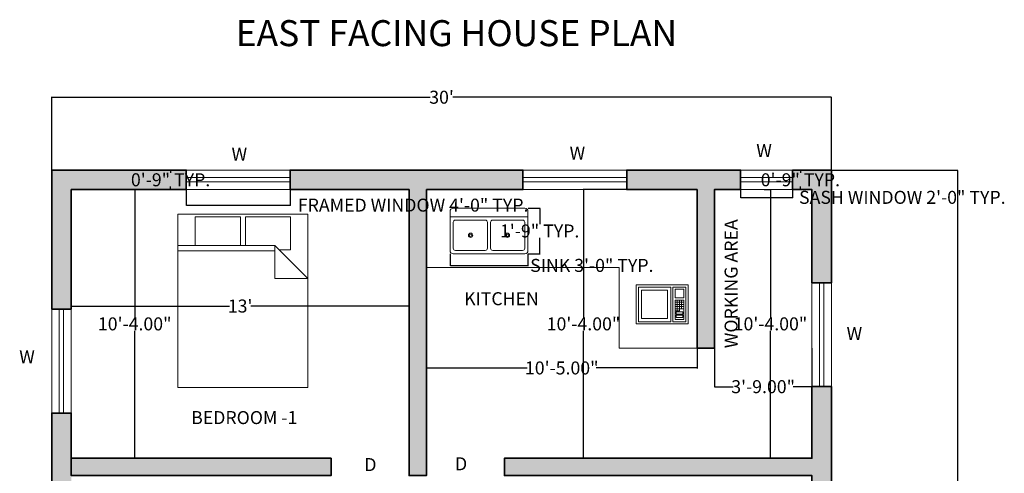
# Model space of a CAD drawing. Units: inches. Extents: x -977 to 1065, y -406 to 125.
# Tile 4 of 4: x 610 to 1065, y -89 to 121. Entities that reach past the tile are written whole.
import ezdxf

# ---------------------------------------------------------------- set-up
doc = ezdxf.new("R2010")
doc.units = ezdxf.units.IN
doc.header["$MEASUREMENT"] = 0
for name, color, linetype, lineweight in [('A-ANNO-DIMS', 2, 'Continuous', 13), ('A-ANNO-TEXT', 7, 'Continuous', 18), ('A-ANNO-TITL', 7, 'Continuous', 25), ('A-AREA-IDEN', 7, 'Continuous', 18), ('A-EQPM', 9, 'Continuous', 18), ('A-FLOR-CASE', 8, 'Continuous', 18), ('A-FLOR-FIXT', 8, 'Continuous', 18), ('A-FURN', 8, 'Continuous', 18), ('A-GLAZ', 5, 'Continuous', 18), ('A-WALL', 7, 'Continuous', 35), ('A-WALL-PATT', 252, 'Continuous', 13)]:
    doc.layers.add(name, color=color, linetype=linetype, lineweight=lineweight)
doc.styles.get("Standard").update_dxf_attribs({"font": 'arial.ttf'})
doc.dimstyles.get("Standard").update_dxf_attribs({"dimtxt": 6, "dimasz": 0.18, "dimexe": 0.18, "dimexo": 0.0625, "dimgap": 0.09, "dimtad": 0, "dimtih": 1, "dimtoh": 1, "dimzin": 0, "dimdsep": 46, "dimlunit": 3, "dimtxsty": 'Standard', "dimcen": 0.09, "dimadec": 0, "dimazin": 0, "dimtfac": 1, "dimtofl": 0, "dimtmove": 0, "dimatfit": 3, "dimfxl": 1, "dimtolj": 1, "dimtzin": 0, "dimarcsym": 0})

# ---------------------------------------------------------------- blocks, each defined once
blk = doc.blocks.new('Bed - Queen')
for p, q in [((0, -80.00003), (0, 0)), ((0, 0), (59.99999, 0)), ((59.99999, 0), (59.99999, -80.00003)), ((7.99999, -1.2), (28.79998, -1.2)), ((7.99999, -14.4), (7.99999, -1.2)), ((28.79998, -1.2), (28.79998, -14.4)), ((31.19999, -1.2), (51.99999, -1.2)), ((31.19999, -14.4), (31.19999, -1.2)), ((51.99999, -1.2), (51.99999, -16.4)), ((0, -14.4), (44.8, -14.4)), ((44.8, -16.8), (0, -16.8)), ((59.99999, -29.6), (44.8, -14.4)), ((44.8, -14.4), (44.8, -29.6)), ((51.99999, -16.4), (46.79936, -16.4)), ((44.8, -29.6), (59.99999, -29.6)), ((59.99999, -80.00003), (0, -80.00003))]:
    blk.add_line(p, q)
blk = doc.blocks.new('Sink-double - 36 in top')
for p, q in [((-18, -4), (18, -4)), ((-0.75, -18.5), (-0.75, -6.5)), ((0.75, -6.5), (0.75, -18.5))]:
    blk.add_line(p, q)
for points in [[(-16.5, 0), (16.5, 0)], [(-18, -19.5), (-18, -1.5)], [(18, -1.5), (18, -19.5)], [(-16.5, -18.5), (-16.5, -6.5)], [(-15.5, -5.5), (-1.75, -5.5)], [(1.75, -5.5), (15.5, -5.5)], [(16.5, -6.5), (16.5, -18.5)], [(16.5, -21), (-16.5, -21)], [(-1.75, -19.5), (-15.5, -19.5)], [(15.5, -19.5), (1.75, -19.5)]]:
    blk.add_lwpolyline(points)
for centre, radius in [((-8.5, -12.5), 1), ((-8.5, -12.5), 0.5), ((8.5, -12.5), 1), ((8.5, -12.5), 0.5)]:
    blk.add_circle(centre, radius)
for centre, radius, start, end in [((-16.5, -1.5), 1.5, 90, 180), ((16.5, -1.5), 1.5, 0, 90), ((-15.5, -6.5), 1, 90, 180), ((-1.75, -6.5), 1, 0, 90), ((1.75, -6.5), 1, 90, 180), ((15.5, -6.5), 1, 0, 90), ((-16.5, -19.5), 1.5, 180, 270), ((-15.5, -18.5), 1, 180, 270), ((-1.75, -18.5), 1, 270, 0), ((1.75, -18.5), 1, 180, 270), ((15.5, -18.5), 1, 270, 0), ((16.5, -19.5), 1.5, 270, 0)]:
    blk.add_arc(centre, radius, start, end)
blk = doc.blocks.new('Microwave')
for p, q in [((18, 10), (22, 10)), ((19, 7), (19, 11)), ((20, 11), (20, 7)), ((21, 7), (21, 11)), ((22, 9), (18, 9)), ((18, 8), (22, 8)), ((22, 7), (18, 7)), ((20, 6), (18, 6)), ((19, 6), (19, 7)), ((20, 7), (20, 6))]:
    blk.add_line(p, q)
for points in [[(0, 0), (0, 18), (24, 18), (24, 0)], [(1, 1), (1, 17), (16, 17), (16, 1)], [(2.5, 2.5), (2.5, 15.5), (14.5, 15.5), (14.5, 2.5)], [(17, 1), (17, 17), (23, 17), (23, 1)], [(18, 12), (18, 16), (22, 16), (22, 12)], [(18, 2), (18, 11), (22, 11), (22, 2)], [(18.5, 4.5), (18.5, 5.5), (21.5, 5.5), (21.5, 4.5)], [(18.5, 3), (18.5, 4), (21.5, 4), (21.5, 3)]]:
    blk.add_lwpolyline(points, close=True)
blk = doc.blocks.new('*D31')
at = {"layer": 'A-ANNO-DIMS', "color": 0, "lineweight": -2, "transparency": 16777216}
for p, q in [((625.09, 51.05), (625.09, 85.12)), ((625.27, 84.94), (799.91, 84.94)), ((984.91, 84.94), (810.27, 84.94)), ((985.09, 51.4), (985.09, 85.12))]:
    blk.add_line(p, q, dxfattribs=at)
at = {"layer": 'A-ANNO-DIMS', "color": 0, "transparency": 16777216}
for points in [[(625.27, 84.97), (625.27, 84.91), (625.09, 84.94)], [(984.91, 84.97), (984.91, 84.91), (985.09, 84.94)]]:
    blk.add_solid(points, dxfattribs=at)
at = {"layer": 'Defpoints', "color": 0, "transparency": 16777216}
for p in [(985.09, 84.94), (625.09, 50.99), (985.09, 51.33)]:
    blk.add_point(p, dxfattribs=at)
at = {"layer": 'A-ANNO-DIMS', "color": 0, "transparency": 16777216, "insert": (805.09, 84.94), "char_height": 6, "attachment_point": 5}
blk.add_mtext("\\A1;30'", dxfattribs=at)
blk = doc.blocks.new('*D32')
at = {"layer": 'A-ANNO-DIMS', "color": 0, "lineweight": -2, "transparency": 16777216}
for p, q in [((985.15, 51.33), (1043.56, 51.33)), ((1043.38, 51.15), (1043.38, -167.51)), ((1043.38, -392.49), (1043.38, -173.82)), ((985.15, -392.67), (1043.56, -392.67))]:
    blk.add_line(p, q, dxfattribs=at)
at = {"layer": 'A-ANNO-DIMS', "color": 0, "transparency": 16777216}
for points in [[(1043.35, 51.15), (1043.41, 51.15), (1043.38, 51.33)], [(1043.35, -392.49), (1043.41, -392.49), (1043.38, -392.67)]]:
    blk.add_solid(points, dxfattribs=at)
at = {"layer": 'Defpoints', "color": 0, "transparency": 16777216}
for p in [(985.09, 51.33), (985.09, -392.67), (1043.38, -392.67)]:
    blk.add_point(p, dxfattribs=at)
at = {"layer": 'A-ANNO-DIMS', "color": 0, "transparency": 16777216, "insert": (1043.38, -170.67), "char_height": 6, "attachment_point": 5}
blk.add_mtext("\\A1;37'", dxfattribs=at)
blk = doc.blocks.new('*D33')
at = {"layer": 'A-ANNO-DIMS', "color": 0, "lineweight": -2, "transparency": 16777216}
for p, q in [((634.09, -3.08), (634.09, -11.62)), ((790.09, -3.08), (790.09, -11.62)), ((634.27, -11.44), (707.19, -11.44)), ((789.91, -11.44), (716.99, -11.44))]:
    blk.add_line(p, q, dxfattribs=at)
at = {"layer": 'A-ANNO-DIMS', "color": 0, "transparency": 16777216}
for points in [[(634.27, -11.41), (634.27, -11.47), (634.09, -11.44)], [(789.91, -11.41), (789.91, -11.47), (790.09, -11.44)]]:
    blk.add_solid(points, dxfattribs=at)
at = {"layer": 'Defpoints', "color": 0, "transparency": 16777216}
for p in [(634.09, -3.02), (790.09, -3.02), (790.09, -11.44)]:
    blk.add_point(p, dxfattribs=at)
at = {"layer": 'A-ANNO-DIMS', "color": 0, "transparency": 16777216, "insert": (712.09, -11.44), "char_height": 6, "attachment_point": 5}
blk.add_mtext("\\A1;13'", dxfattribs=at)
blk = doc.blocks.new('*D34')
at = {"layer": 'A-ANNO-DIMS', "color": 0, "lineweight": -2, "transparency": 16777216}
for p, q in [((668.37, 42.33), (663.23, 42.33)), ((663.41, 42.15), (663.41, -16.51)), ((663.41, -81.49), (663.41, -22.82)), ((668.37, -81.67), (663.23, -81.67))]:
    blk.add_line(p, q, dxfattribs=at)
at = {"layer": 'A-ANNO-DIMS', "color": 0, "transparency": 16777216}
for points in [[(663.38, 42.15), (663.44, 42.15), (663.41, 42.33)], [(663.38, -81.49), (663.44, -81.49), (663.41, -81.67)]]:
    blk.add_solid(points, dxfattribs=at)
at = {"layer": 'Defpoints', "color": 0, "transparency": 16777216}
for p in [(668.43, 42.33), (663.41, -81.67), (668.43, -81.67)]:
    blk.add_point(p, dxfattribs=at)
at = {"layer": 'A-ANNO-DIMS', "color": 0, "transparency": 16777216, "insert": (663.41, -19.67), "char_height": 6, "attachment_point": 5}
blk.add_mtext('\\A1;10\'-4.00"', dxfattribs=at)
blk = doc.blocks.new('*D37')
at = {"layer": 'A-ANNO-DIMS', "color": 0, "lineweight": -2, "transparency": 16777216}
for p, q in [((798.09, 6.27), (798.09, -40.2)), ((923.09, 5.65), (923.09, -40.2)), ((798.27, -40.02), (844.65, -40.02)), ((922.91, -40.02), (876.53, -40.02))]:
    blk.add_line(p, q, dxfattribs=at)
at = {"layer": 'A-ANNO-DIMS', "color": 0, "transparency": 16777216}
for points in [[(798.27, -39.99), (798.27, -40.05), (798.09, -40.02)], [(922.91, -39.99), (922.91, -40.05), (923.09, -40.02)]]:
    blk.add_solid(points, dxfattribs=at)
at = {"layer": 'Defpoints', "color": 0, "transparency": 16777216}
for p in [(798.09, 6.33), (923.09, 5.72), (923.09, -40.02)]:
    blk.add_point(p, dxfattribs=at)
at = {"layer": 'A-ANNO-DIMS', "color": 0, "transparency": 16777216, "insert": (860.59, -40.02), "char_height": 6, "attachment_point": 5}
blk.add_mtext('\\A1;10\'-5.00"', dxfattribs=at)
blk = doc.blocks.new('*D38')
at = {"layer": 'A-ANNO-DIMS', "color": 0, "lineweight": -2, "transparency": 16777216}
for p, q in [((901.19, 42.33), (870.46, 42.33)), ((870.64, 42.15), (870.64, -16.51)), ((870.64, -81.49), (870.64, -22.82)), ((901.19, -81.67), (870.46, -81.67))]:
    blk.add_line(p, q, dxfattribs=at)
at = {"layer": 'A-ANNO-DIMS', "color": 0, "transparency": 16777216}
for points in [[(870.61, 42.15), (870.67, 42.15), (870.64, 42.33)], [(870.61, -81.49), (870.67, -81.49), (870.64, -81.67)]]:
    blk.add_solid(points, dxfattribs=at)
at = {"layer": 'Defpoints', "color": 0, "transparency": 16777216}
for p in [(901.25, 42.33), (870.64, -81.67), (901.25, -81.67)]:
    blk.add_point(p, dxfattribs=at)
at = {"layer": 'A-ANNO-DIMS', "color": 0, "transparency": 16777216, "insert": (870.64, -19.67), "char_height": 6, "attachment_point": 5}
blk.add_mtext('\\A1;10\'-4.00"', dxfattribs=at)
blk = doc.blocks.new('*D39')
at = {"layer": 'A-ANNO-DIMS', "color": 0, "lineweight": -2, "transparency": 16777216}
for p, q in [((954.03, 42.33), (957.16, 42.33)), ((956.98, 42.15), (956.98, -16.51)), ((956.98, -81.49), (956.98, -22.82)), ((954.03, -81.67), (957.16, -81.67))]:
    blk.add_line(p, q, dxfattribs=at)
at = {"layer": 'A-ANNO-DIMS', "color": 0, "transparency": 16777216}
for points in [[(956.95, 42.15), (957.01, 42.15), (956.98, 42.33)], [(956.95, -81.49), (957.01, -81.49), (956.98, -81.67)]]:
    blk.add_solid(points, dxfattribs=at)
at = {"layer": 'Defpoints', "color": 0, "transparency": 16777216}
for p in [(953.97, 42.33), (953.97, -81.67), (956.98, -81.67)]:
    blk.add_point(p, dxfattribs=at)
at = {"layer": 'A-ANNO-DIMS', "color": 0, "transparency": 16777216, "insert": (956.98, -19.67), "char_height": 6, "attachment_point": 5}
blk.add_mtext('\\A1;10\'-4.00"', dxfattribs=at)
blk = doc.blocks.new('*D40')
at = {"layer": 'A-ANNO-DIMS', "color": 0, "lineweight": -2, "transparency": 16777216}
for p, q in [((931.09, -30.96), (931.09, -48.84)), ((976.09, -30.96), (976.09, -48.84)), ((931.27, -48.66), (939.7, -48.66)), ((975.91, -48.66), (967.48, -48.66))]:
    blk.add_line(p, q, dxfattribs=at)
at = {"layer": 'A-ANNO-DIMS', "color": 0, "transparency": 16777216}
for points in [[(931.27, -48.63), (931.27, -48.69), (931.09, -48.66)], [(975.91, -48.63), (975.91, -48.69), (976.09, -48.66)]]:
    blk.add_solid(points, dxfattribs=at)
at = {"layer": 'Defpoints', "color": 0, "transparency": 16777216}
for p in [(931.09, -30.9), (976.09, -30.9), (976.09, -48.66)]:
    blk.add_point(p, dxfattribs=at)
at = {"layer": 'A-ANNO-DIMS', "color": 0, "transparency": 16777216, "insert": (953.59, -48.66), "char_height": 6, "attachment_point": 5}
blk.add_mtext('\\A1;3\'-9.00"', dxfattribs=at)
blk = doc.blocks.new('WIN-48-FRAMED')
for p, q in [((0, 48), (9, 48)), ((0, 0), (0, 48)), ((3.5, 0), (3.5, 48)), ((5.5, 48), (5.5, 0)), ((9, 48), (9, 0)), ((9, 0), (0, 0))]:
    blk.add_line(p, q)
for points in [[(0, 0), (0, 48)], [(9, 0), (9, 48)]]:
    blk.add_lwpolyline(points)
blk = doc.blocks.new('WIN-24-SASH')
for p, q in [((0, 5.5), (24, 5.5)), ((24, 9), (24, 0)), ((24, 3.5), (0, 3.5)), ((24, 0), (0, 0))]:
    blk.add_line(p, q)
for points in [[(0, 9), (24, 9)], [(0, 0), (24, 0)]]:
    blk.add_lwpolyline(points)
blk = doc.blocks.new('*D52')
at = {"layer": 'A-ANNO-DIMS', "color": 0, "lineweight": -2, "transparency": 16777216}
for p, q in [((687.18, 42.27), (687.18, 34.95)), ((735.18, 42.27), (735.18, 34.95)), ((687.36, 35.13), (735, 35.13)), ((735.18, 35.13), (735.36, 35.13))]:
    blk.add_line(p, q, dxfattribs=at)
at = {"layer": 'A-ANNO-DIMS', "color": 0, "transparency": 16777216}
for points in [[(687.36, 35.16), (687.36, 35.1), (687.18, 35.13)], [(735, 35.16), (735, 35.1), (735.18, 35.13)]]:
    blk.add_solid(points, dxfattribs=at)
at = {"layer": 'Defpoints', "color": 0, "transparency": 16777216}
for p in [(687.18, 42.33), (735.18, 42.33), (735.18, 35.13)]:
    blk.add_point(p, dxfattribs=at)
at = {"layer": 'A-ANNO-DIMS', "color": 0, "transparency": 16777216, "insert": (791.98, 35.13), "char_height": 6, "attachment_point": 5}
blk.add_mtext('\\A1;FRAMED WINDOW 4\'-0" TYP.', dxfattribs=at)
blk = doc.blocks.new('*D53')
at = {"layer": 'A-ANNO-DIMS', "color": 0, "lineweight": -2, "transparency": 16777216}
for p, q in [((687.12, 51.33), (679.8, 51.33)), ((679.98, 51.15), (679.98, 49.99)), ((687.12, 42.33), (679.8, 42.33)), ((679.98, 42.51), (679.98, 43.68))]:
    blk.add_line(p, q, dxfattribs=at)
at = {"layer": 'A-ANNO-DIMS', "color": 0, "transparency": 16777216}
for points in [[(679.95, 51.15), (680.01, 51.15), (679.98, 51.33)], [(679.95, 42.51), (680.01, 42.51), (679.98, 42.33)]]:
    blk.add_solid(points, dxfattribs=at)
at = {"layer": 'Defpoints', "color": 0, "transparency": 16777216}
for p in [(687.18, 51.33), (679.98, 42.33), (687.18, 42.33)]:
    blk.add_point(p, dxfattribs=at)
at = {"layer": 'A-ANNO-DIMS', "color": 0, "transparency": 16777216, "insert": (679.98, 46.83), "char_height": 6, "attachment_point": 5}
blk.add_mtext('\\A1;0\'-9" TYP.', dxfattribs=at)
blk = doc.blocks.new('*D58')
at = {"layer": 'A-ANNO-DIMS', "color": 0, "lineweight": -2, "transparency": 16777216}
for p, q in [((943.18, 42.27), (943.18, 38.55)), ((967.18, 42.27), (967.18, 38.55)), ((943.36, 38.73), (967, 38.73)), ((967.18, 38.73), (967.36, 38.73))]:
    blk.add_line(p, q, dxfattribs=at)
at = {"layer": 'A-ANNO-DIMS', "color": 0, "transparency": 16777216}
for points in [[(943.36, 38.76), (943.36, 38.7), (943.18, 38.73)], [(967, 38.76), (967, 38.7), (967.18, 38.73)]]:
    blk.add_solid(points, dxfattribs=at)
at = {"layer": 'Defpoints', "color": 0, "transparency": 16777216}
for p in [(943.18, 42.33), (967.18, 42.33), (967.18, 38.73)]:
    blk.add_point(p, dxfattribs=at)
at = {"layer": 'A-ANNO-DIMS', "color": 0, "transparency": 16777216, "insert": (1017.85, 38.73), "char_height": 6, "attachment_point": 5}
blk.add_mtext('\\A1;SASH WINDOW 2\'-0" TYP.', dxfattribs=at)
blk = doc.blocks.new('*D59')
at = {"layer": 'A-ANNO-DIMS', "color": 0, "lineweight": -2, "transparency": 16777216}
for p, q in [((967.24, 51.33), (970.96, 51.33)), ((970.78, 51.15), (970.78, 49.99)), ((967.24, 42.33), (970.96, 42.33)), ((970.78, 42.51), (970.78, 43.68))]:
    blk.add_line(p, q, dxfattribs=at)
at = {"layer": 'A-ANNO-DIMS', "color": 0, "transparency": 16777216}
for points in [[(970.75, 51.15), (970.81, 51.15), (970.78, 51.33)], [(970.75, 42.51), (970.81, 42.51), (970.78, 42.33)]]:
    blk.add_solid(points, dxfattribs=at)
at = {"layer": 'Defpoints', "color": 0, "transparency": 16777216}
for p in [(967.18, 51.33), (970.78, 51.33), (967.18, 42.33)]:
    blk.add_point(p, dxfattribs=at)
at = {"layer": 'A-ANNO-DIMS', "color": 0, "transparency": 16777216, "insert": (970.78, 46.83), "char_height": 6, "attachment_point": 5}
blk.add_mtext('\\A1;0\'-9" TYP.', dxfattribs=at)
blk = doc.blocks.new('*D60')
at = {"layer": 'A-ANNO-DIMS', "color": 0, "lineweight": -2, "transparency": 16777216}
for p, q in [((809.01, 12.65), (809.01, 7.13)), ((845.01, 12.65), (845.01, 7.13)), ((809.19, 7.31), (844.83, 7.31)), ((845.01, 7.31), (845.19, 7.31))]:
    blk.add_line(p, q, dxfattribs=at)
at = {"layer": 'A-ANNO-DIMS', "color": 0, "transparency": 16777216}
for points in [[(809.19, 7.34), (809.19, 7.28), (809.01, 7.31)], [(844.83, 7.34), (844.83, 7.28), (845.01, 7.31)]]:
    blk.add_solid(points, dxfattribs=at)
at = {"layer": 'Defpoints', "color": 0, "transparency": 16777216}
for p in [(809.01, 12.71), (845.01, 12.71), (845.01, 7.31)]:
    blk.add_point(p, dxfattribs=at)
at = {"layer": 'A-ANNO-DIMS', "color": 0, "transparency": 16777216, "insert": (874.5, 7.31), "char_height": 6, "attachment_point": 5}
blk.add_mtext('\\A1;SINK 3\'-0" TYP.', dxfattribs=at)
blk = doc.blocks.new('*D61')
at = {"layer": 'A-ANNO-DIMS', "color": 0, "lineweight": -2, "transparency": 16777216}
for p, q in [((845.07, 33.71), (850.59, 33.71)), ((850.41, 33.53), (850.41, 26.36)), ((850.41, 12.89), (850.41, 20.06)), ((845.07, 12.71), (850.59, 12.71))]:
    blk.add_line(p, q, dxfattribs=at)
at = {"layer": 'A-ANNO-DIMS', "color": 0, "transparency": 16777216}
for points in [[(850.38, 33.53), (850.44, 33.53), (850.41, 33.71)], [(850.38, 12.89), (850.44, 12.89), (850.41, 12.71)]]:
    blk.add_solid(points, dxfattribs=at)
at = {"layer": 'Defpoints', "color": 0, "transparency": 16777216}
for p in [(845.01, 33.71), (850.41, 33.71), (845.01, 12.71)]:
    blk.add_point(p, dxfattribs=at)
at = {"layer": 'A-ANNO-DIMS', "color": 0, "transparency": 16777216, "insert": (850.41, 23.21), "char_height": 6, "attachment_point": 5}
blk.add_mtext('\\A1;1\'-9" TYP.', dxfattribs=at)

msp = doc.modelspace()

# ---------------------------------------------------------------- hatches: boundary and pattern name
at = {"layer": 'A-WALL-PATT'}
h = msp.add_hatch(color=256, dxfattribs=at)
h.dxf.hatch_style = 1
h.paths.add_polyline_path([(637.06, 42.333), (687.18, 42.333), (687.18, 51.333), (625.089, 51.333), (625.089, -12.85), (634.089, -12.85), (634.089, 42.333)])
h = msp.add_hatch(color=256, dxfattribs=at)
h.dxf.hatch_style = 1
h.paths.add_polyline_path([(798.089, 42.333), (798.089, -89.667), (790.089, -89.667), (790.089, 42.333), (735.18, 42.333), (735.18, 51.333), (842.634, 51.333), (842.634, 42.333)])
h = msp.add_hatch(color=256, dxfattribs=at)
h.dxf.hatch_style = 1
h.paths.add_polyline_path([(943.182, 42.333), (943.182, 51.333), (890.634, 51.333), (890.634, 42.333), (923.089, 42.333), (923.089, -30.9), (931.089, -30.9), (931.089, 42.333)])
h = msp.add_hatch(color=256, dxfattribs=at)
h.dxf.hatch_style = 1
h.paths.add_polyline_path([(985.089, -0.655), (985.089, 51.333), (967.182, 51.333), (967.182, 42.333), (976.089, 42.333), (976.089, -0.655)])
h = msp.add_hatch(color=256, dxfattribs=at)
h.dxf.hatch_style = 1
h.paths.add_polyline_path([(985.089, -125.667), (985.089, -48.655), (976.089, -48.655), (976.089, -81.667), (834.089, -81.667), (834.089, -89.667), (976.089, -89.667), (976.089, -125.667)])
h = msp.add_hatch(color=256, dxfattribs=at)
h.dxf.hatch_style = 1
h.paths.add_polyline_path([(625.089, -109.279), (625.089, -60.85), (634.089, -60.85), (634.089, -109.279)])
h = msp.add_hatch(color=256, dxfattribs=at)
h.dxf.hatch_style = 1
h.paths.add_polyline_path([(754.089, -81.667), (634.089, -81.667), (634.089, -89.667), (754.089, -89.667)])

# ---------------------------------------------------------------- linework, layer by layer
at = {"layer": 'A-FLOR-CASE'}
msp.add_line((887.089, -30.9), (923.089, -30.9), dxfattribs=at)
for points in [[(798.089, 6.333), (887.089, 6.333)], [(887.089, -30.9), (887.089, 6.333)]]:
    msp.add_lwpolyline(points, dxfattribs=at)
at = {"layer": 'A-GLAZ'}
for p, q in [((943.182, 51.333), (967.182, 51.333)), ((735.18, 42.333), (735.18, 46.833))]:
    msp.add_line(p, q, dxfattribs=at)
at = {"layer": 'A-WALL'}
for points in [[(637.06, 42.333), (687.18, 42.333), (687.18, 51.333), (625.089, 51.333), (625.089, -12.85), (634.089, -12.85), (634.089, 42.333)], [(798.089, 42.333), (798.089, -89.667), (790.089, -89.667), (790.089, 42.333), (735.18, 42.333), (735.18, 51.333), (842.634, 51.333), (842.634, 42.333)], [(943.182, 42.333), (943.182, 51.333), (890.634, 51.333), (890.634, 42.333), (923.089, 42.333), (923.089, -30.9), (931.089, -30.9), (931.089, 42.333)], [(985.089, -0.655), (985.089, 51.333), (967.182, 51.333), (967.182, 42.333), (976.089, 42.333), (976.089, -0.655)], [(754.089, -81.667), (634.089, -81.667), (634.089, -89.667), (754.089, -89.667)]]:
    msp.add_lwpolyline(points, close=True, dxfattribs=at)
for points in [[(985.089, -125.667), (985.089, -48.655), (976.089, -48.655), (976.089, -81.667), (834.089, -81.667), (834.089, -89.667), (976.089, -89.667), (976.089, -125.667), (985.089, -125.667), (985.089, -116.301)], [(625.089, -109.279), (625.089, -60.85), (634.089, -60.85), (634.089, -81.667)]]:
    msp.add_lwpolyline(points, dxfattribs=at)

# ---------------------------------------------------------------- block references
at = {"layer": 'A-EQPM'}
msp.add_blockref('Microwave', (894.96, -19.685), dxfattribs=at)
at = {"layer": 'A-FLOR-FIXT'}
msp.add_blockref('Sink-double - 36 in top', (827.01, 33.711), dxfattribs=at)
at = {"layer": 'A-FURN'}
msp.add_blockref('Bed - Queen', (683.391, 30.912), dxfattribs=at)
at = {"layer": 'A-GLAZ'}
for p, rotation in [((687.18, 51.333), 269.9999999999999), ((842.634, 51.333), 270), ((985.089, -0.655), 180)]:
    msp.add_blockref('WIN-48-FRAMED', p, dxfattribs=dict(at, rotation=rotation))
for name, p in [('WIN-24-SASH', (943.182, 42.333)), ('WIN-48-FRAMED', (625.089, -60.85))]:
    msp.add_blockref(name, p, dxfattribs=at)

# ---------------------------------------------------------------- texts
at = {"layer": 'A-ANNO-TEXT', "char_height": 6, "attachment_point": 1}
for s, insert in [('W ', (708.137, 61.625)), ('W ', (864.218, 62.188)), ('W ', (950.428, 63.314)), ('W ', (992.125, -21.14)), ('W ', (610.094, -31.837)), ('D ', (769.431, -81.617)), ('D ', (811.31, -81.26))]:
    msp.add_mtext_dynamic_manual_height_columns(s, width=77.77408, gutter_width=1, heights=[0], dxfattribs=dict(at, insert=insert))
at = {"layer": 'A-ANNO-TITL', "insert": (710.034, 120.507), "char_height": 12, "attachment_point": 1}
msp.add_mtext_dynamic_manual_height_columns('EAST FACING HOUSE PLAN ', width=255.23349, gutter_width=1, heights=[0], dxfattribs=at)
at = {"layer": 'A-AREA-IDEN', "insert": (935.804, -30.9), "char_height": 6, "attachment_point": 1, "rotation": 90}
msp.add_mtext_dynamic_manual_height_columns('WORKING AREA', width=77.77408, gutter_width=1, heights=[0], dxfattribs=at)
at = {"layer": 'A-AREA-IDEN', "char_height": 6, "attachment_point": 1}
for s, insert in [('KITCHEN', (815.509, -5.047)), ('BEDROOM -1', (689.464, -59.931))]:
    msp.add_mtext_dynamic_manual_height_columns(s, width=77.77408, gutter_width=1, heights=[0], dxfattribs=dict(at, insert=insert))

# ---------------------------------------------------------------- dimensions: what is measured, and where the dimension line sits
at = {"layer": 'A-ANNO-DIMS'}
for base, p1, p2, picture, middle in [((985.089, 84.943), (625.089, 50.987), (985.089, 51.333), '*D31', (805.089, 84.943)), ((923.089, -40.015), (798.089, 6.333), (923.089, 5.716), '*D37', (860.589, -40.015)), ((790.089, -11.436), (634.089, -3.021), (790.089, -3.021), '*D33', (712.089, -11.436)), ((976.089, -48.655), (931.089, -30.9), (976.089, -30.9), '*D40', (953.589, -48.655))]:
    dim = msp.add_linear_dim(base=base, p1=p1, p2=p2, dimstyle='Standard', override={"dimclrd": 0, "dimclre": 0, "dimclrt": 0}, dxfattribs=at)
    dim.commit()
    dim.dimension.update_dxf_attribs({"geometry": picture, "text_midpoint": middle})
for base, p1, p2, angle, picture, middle in [((679.98, 42.333), (687.18, 51.333), (687.18, 42.333), 270, '*D53', (679.98, 46.833)), ((970.782, 51.333), (967.182, 42.333), (967.182, 51.333), 90, '*D59', (970.782, 46.833)), ((850.41, 33.711), (845.01, 12.711), (845.01, 33.711), 90, '*D61', (850.41, 23.211))]:
    dim = msp.add_linear_dim(base=base, p1=p1, p2=p2, angle=angle, text='<> TYP.', dimstyle='Standard', override={"dimdec": 1, "dimlfac": 1, "dimrnd": 0, "dimzin": 1, "dimdsep": 46, "dimlunit": 4, "dimfrac": 2}, dxfattribs=at)
    dim.commit()
    dim.dimension.update_dxf_attribs({"geometry": picture, "text_midpoint": middle})
for base, p1, p2, text, picture, middle in [((967.182, 38.733), (943.182, 42.333), (967.182, 42.333), 'SASH WINDOW <> TYP.', '*D58', (1017.855, 38.733)), ((735.18, 35.133), (687.18, 42.333), (735.18, 42.333), 'FRAMED WINDOW <> TYP.', '*D52', (791.98, 35.133)), ((845.01, 7.311), (809.01, 12.711), (845.01, 12.711), 'SINK <> TYP.', '*D60', (874.499, 7.311))]:
    dim = msp.add_linear_dim(base=base, p1=p1, p2=p2, text=text, dimstyle='Standard', override={"dimdec": 1, "dimlfac": 1, "dimrnd": 0, "dimzin": 1, "dimdsep": 46, "dimlunit": 4, "dimfrac": 2}, dxfattribs=at)
    dim.commit()
    dim.dimension.update_dxf_attribs({"geometry": picture, "text_midpoint": middle})
for base, p1, p2, picture, middle in [((1043.377, -392.667), (985.089, 51.333), (985.089, -392.667), '*D32', (1043.377, -170.667)), ((663.412, -81.667), (668.429, 42.333), (668.429, -81.667), '*D34', (663.412, -19.667)), ((870.644, -81.667), (901.252, 42.333), (901.252, -81.667), '*D38', (870.644, -19.667)), ((956.981, -81.667), (953.97, 42.333), (953.97, -81.667), '*D39', (956.981, -19.667))]:
    dim = msp.add_linear_dim(base=base, p1=p1, p2=p2, angle=90, dimstyle='Standard', override={"dimclrd": 0, "dimclre": 0, "dimclrt": 0}, dxfattribs=at)
    dim.commit()
    dim.dimension.update_dxf_attribs({"geometry": picture, "text_midpoint": middle})

doc.saveas('drawing.dxf')
